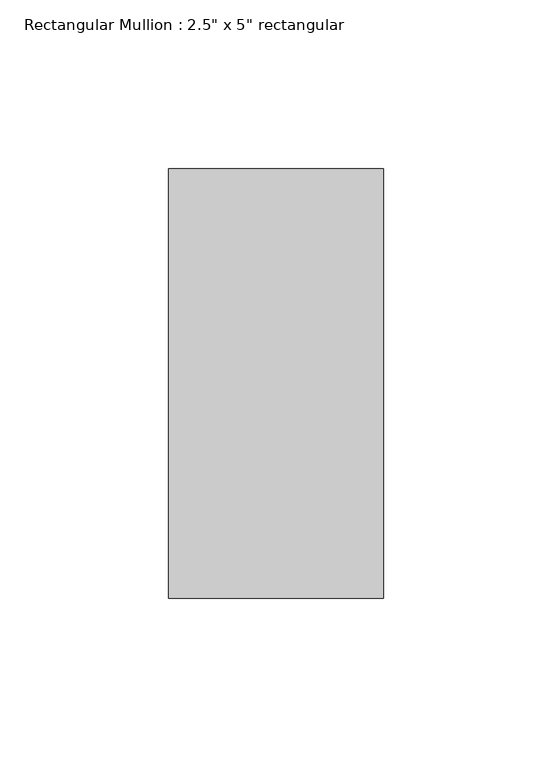
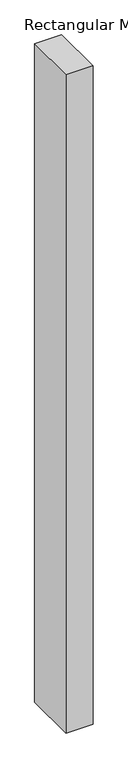
"""IFC4 building model written with IfcOpenShell, lengths in millimetres: member geometry."""

from ifc_helpers import new_model, si_unit, frame, origin, place, context, project, spatial, polyline, outline, extrude, source, transform, mapped, element, save


def member_11644e99(model_context):
    return source(origin(), model_context, "Body", "SweptSolid", [
        extrude(outline(polyline([(31.75, 63.5), (31.75, -63.5), (-31.75, -63.5), (-31.75, 63.5), (31.75, 63.5)])), frame((0.0, 0.0, -1631.45108), z_axis=(0.0, 0.0, 1.0), x_axis=(1.0, 0.0, 0.0)), (0.0, 0.0, 1.0), 1631.45108),
    ])


if __name__ == "__main__":
    model = new_model("IFC4")
    model_context = context("Model", 3, world=origin())
    ifc_project = project(units=[si_unit("LENGTHUNIT", "METRE", prefix="MILLI")], contexts=[model_context])
    site = spatial("IfcSite", under=ifc_project)
    building = spatial("IfcBuilding", under=site)
    placement = place(None, origin())
    member_shape = member_11644e99(model_context)
    element("IfcMember", 1, ObjectType="Rectangular Mullion : 2.5\" x 5\" rectangular", at=placement, inside=building, context=model_context, shape_type="MappedRepresentation", body=[
        mapped(member_shape, transform((0.0, 0.0, 0.0), x_axis=(1.0, 0.0, 0.0), y_axis=(0.0, 1.0, 0.0), z_axis=(0.0, 0.0, 1.0))),
    ])
    save(model, "model.ifc")

# Revit data of these elements
# Type "Rectangular Mullion : 2.5\" x 5\" rectangular"
#   built-in parameter 1007304 = 0.416667 (stored number, unit not read)
#   built-in parameter 1007301 = 0.104167 (stored number, unit not read)
#   built-in parameter 1007300 = 0.104167 (stored number, unit not read)
# Element 1 (IfcMember, "Rectangular Mullion : 2.5\" x 5\" rectangular")
#   Materials on its faces: "Aluminum"
# Materials
#   "Aluminum": class "Metal", colour RGB 247 247 247, transparency 0, Description = "Aluminum 6061", Cost = 0
